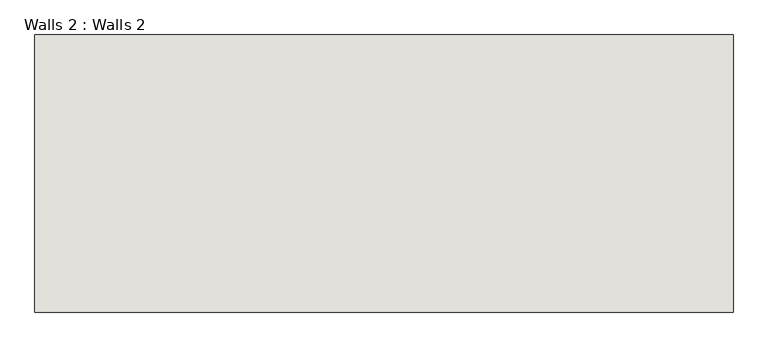
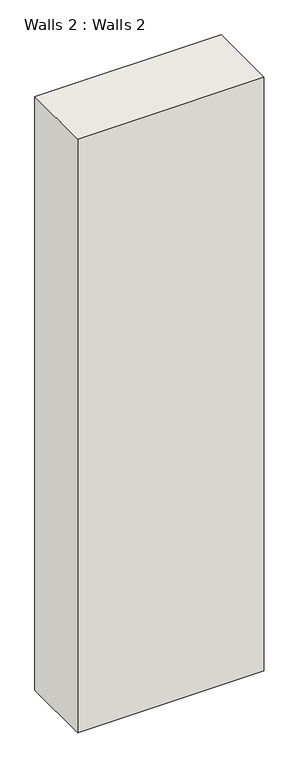
"""IFC4 building model written with IfcOpenShell, lengths in millimetres: wall geometry, Walls 2 : Walls 2."""

from ifc_helpers import new_model, si_unit, frame, origin, place, context, project, spatial, polyline, outline, extrude, source, transform, mapped, element, save


def walls_2_walls_2_595a3e20(model_context):
    return source(origin(), model_context, "Body", "SweptSolid", [
        extrude(outline(polyline([(-5606.7936733, 3506.5419215), (-8705.5936733, 3506.5419215), (-8705.5936733, 4738.4419215), (-5606.7936733, 4738.4419215), (-5606.7936733, 3506.5419215)])), frame((0.0, 0.0, 2347.5273004), z_axis=(0.0, 0.0, 1.0), x_axis=(1.0, 0.0, 0.0)), (0.0, 0.0, 1.0), 10454.0726996),
    ])


if __name__ == "__main__":
    model = new_model("IFC4")
    model_context = context("Model", 3, world=origin())
    ifc_project = project(units=[si_unit("LENGTHUNIT", "METRE", prefix="MILLI")], contexts=[model_context])
    site = spatial("IfcSite", under=ifc_project)
    building = spatial("IfcBuilding", under=site)
    placement = place(None, origin())
    walls_2_walls_2_shape = walls_2_walls_2_595a3e20(model_context)
    element("IfcWall", 1, ObjectType="Walls 2 : Walls 2", at=placement, inside=building, context=model_context, shape_type="MappedRepresentation", body=[
        mapped(walls_2_walls_2_shape, transform((0.0, 0.0, 0.0), x_axis=(1.0, 0.0, 0.0), y_axis=(0.0, 1.0, 0.0), z_axis=(0.0, 0.0, 1.0))),
    ])
    save(model, "model.ifc")

# Revit data of these elements
# Element 1 (IfcWall, "Walls 2 : Walls 2")
#   Materials on its faces: "Default Wall"
# Materials
#   "Default Wall": colour RGB 128 128 128, transparency 0
